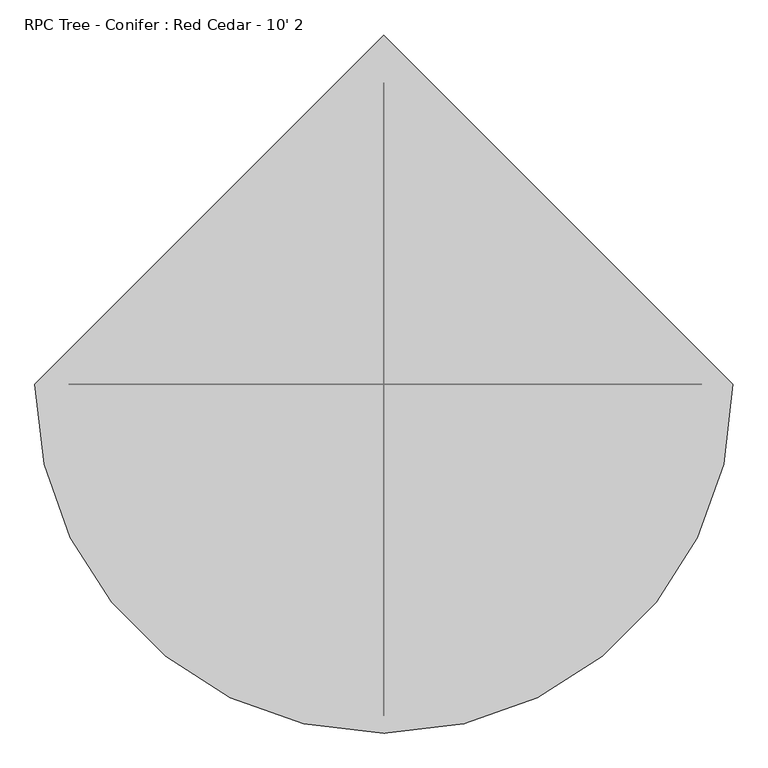
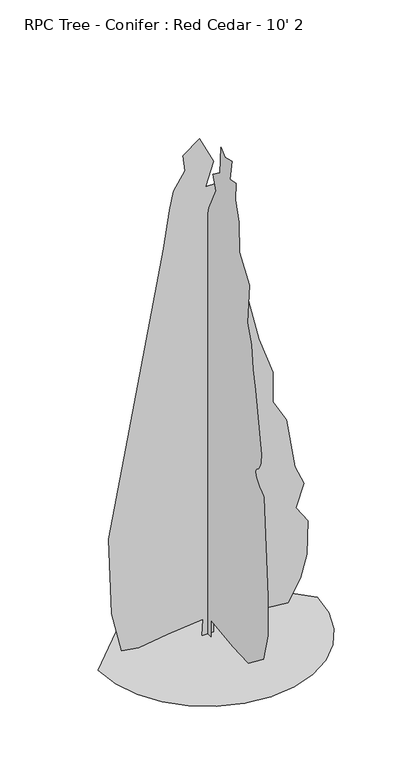
"""IFC4 building model written with IfcOpenShell, lengths in millimetres: geographic element geometry, RPC Tree - Conifer : Red Cedar - 10' 2."""

from ifc_helpers import new_model, si_unit, origin, place, context, project, spatial, triangles, source, transform, mapped, element, save


def rpc_tree_conifer_red_cedar_10_2_15f97043(model_context):
    return source(origin(), model_context, "Body", "Tessellation", [
        triangles([(-83.5718611, 3.7e-06, 7.4e-06), (-70.6343741, -1.16e-05, 245.8064897), (-584.0888028, 1.37e-05, 198.451386), (-999.4580349, 3.55e-05, 137.2780578), (-1247.914381, 4.38e-05, 181.12034), (-1390.2241539, 1.37e-05, 789.1649843), (-1429.0354477, -5.32e-05, 1940.5782063), (-1209.1032326, -0.0001322, 3104.9200722), (-639.8703907, -0.0003352, 6093.4065536), (-549.3098574, -0.0003723, 6649.7173645), (-497.5611992, -0.0003908, 6921.3699692), (-329.3777149, -0.0004136, 7180.132663), (-355.252044, -0.0004263, 7412.9870544), (-122.3830459, -0.0004473, 7594.1527405), (84.6116323, -0.0004317, 7180.132663), (-31.8227487, -0.0004057, 6830.819101), (123.4234529, -0.0004125, 6830.819101), (739.2029903, -0.0002848, 4235.9626625), (938.4659002, -0.0002592, 3661.2180931), (938.4659002, -0.0002322, 3208.4186966), (1132.5218605, -0.0002207, 2872.0531815), (1261.8966671, -0.0001808, 2108.7579117), (1391.2652241, -0.0001688, 1811.2033997), (1274.8316334, -0.0001436, 1474.8377392), (1443.0177338, -0.0001356, 1216.0943756), (1430.0763725, -0.0001049, 711.5426147), (1339.5191093, -8.09e-05, 375.1781533), (1158.3981153, -5.45e-05, 64.6861543), (855.0587093, -4.33e-05, 100.3528226), (433.9154838, -2.44e-05, 90.5604879), (84.6116323, -1.68e-05, 219.9321606), (84.6116323, -3.7e-06, 0.0), (0.1966743, 73.339932, 0.0002301), (0.1966695, 99.2142657, 181.1209758), (0.1966868, 295.5352312, 63.0784626), (0.1966932, 655.5102064, 168.1834843), (0.1966943, 577.8897626, 271.680837), (0.1967153, 1056.5633429, 271.680837), (0.1967266, 1263.5606644, 323.4294951), (0.1967413, 1302.3718128, 620.9846975), (0.196754, 1367.0591434, 1164.3482609), (0.1967591, 1276.4954853, 1371.3391148), (0.1967743, 1289.4368465, 1707.7047752), (0.19678, 1198.8731884, 1927.6369904), (0.1967899, 1160.0619673, 2509.8110481), (0.1967921, 991.8823345, 2729.7432632), (0.1968161, 759.0088308, 3829.4040482), (0.1968294, 500.2661213, 4709.132618), (0.1968359, 319.1464354, 5355.9940063), (0.1968348, 228.5859384, 5420.6755234), (0.1968461, 150.9629329, 5757.0410385), (0.1968576, -30.1575978, 6520.3677017), (0.1968655, -211.2783829, 6882.571756), (0.1968641, -133.6553774, 7089.5817947), (0.1968624, -301.8388799, 7218.9308762), (0.1968788, -327.713209, 7619.9970932), (0.1968703, -431.2105617, 7529.446225), (0.1968647, -599.3933919, 7568.2444382), (0.1968534, -560.5822071, 7270.6835312), (0.1968483, -702.8939421, 7296.5918335), (0.1968375, -689.9526535, 7037.8291397), (0.196835, -780.5163116, 6753.2220932), (0.1968147, -793.4512053, 6300.4038025), (0.1968022, -1047.5908527, 5951.6303238), (0.1967782, -987.5071655, 5343.0529358), (0.1967618, -1091.0057899, 5071.3747513), (0.1967587, -1129.8169384, 4722.0675842), (0.1967434, -1194.5043417, 4437.4544334), (0.1967121, -1336.8141872, 3544.7845024), (0.1967102, -1336.4713303, 3500.4677307), (0.1967083, -1334.0963299, 3456.3733292), (0.1967067, -1327.6448341, 3412.7361671), (0.1967054, -1315.084409, 3369.7786148), (0.1967044, -1294.3770973, 3327.7224609), (0.196704, -1263.4907558, 3286.7967613), (0.1967042, -1220.3805965, 3247.2299904), (0.1967033, -1194.1487675, 3201.3574997), (0.1967003, -1206.8043177, 3145.5030602), (0.196696, -1245.6345783, 3085.8764671), (0.1966912, -1297.9457748, 3028.694783), (0.1966868, -1351.0381737, 2980.155304), (0.1966835, -1392.2051376, 2946.4814873), (0.1966961, -1408.7470058, 2933.8703384), (0.196642, -1504.9938927, 1474.8377392), (0.1966299, -1504.9938927, 879.7286425), (0.1966163, -1388.560302, 452.8011769), (0.1966203, -1013.3834204, 168.1834843), (0.1966378, -625.2671396, 181.12034), (0.1966649, -81.9060743, 258.7433454), (0.1966675, -81.9060743, 0.0002209), (-1583.3149841, 0.0, 0.000295), (-1541.449371, -362.8356654, 0.0002715), (-1422.2281597, -696.0422527, 0.0002465), (-1235.1826, -990.0725613, 0.0002208), (-989.8759163, -1235.379245, 0.0001954), (-695.8456078, -1422.4248047, 0.0001714), (-362.6389841, -1541.6460159, 0.0001497), (0.1967407, -1583.5116291, 0.0001314), (363.0323467, -1541.6460159, 0.000118), (696.2388977, -1422.4248047, 0.0003326), (990.2692062, -1235.379245, 0.0003309), (1235.5822849, -990.0725613, 0.0003348), (1422.6214497, -696.0422527, 0.0001221), (1541.8426609, -362.8356654, 0.0001368), (1583.7082741, 0.0001384, 0.0001566), (0.1964627, 1583.5116291, 0.0003202)], [[13, 14, 15], [12, 13, 15], [12, 15, 16], [11, 12, 16], [32, 1, 2], [31, 32, 2], [10, 11, 16], [16, 17, 18], [10, 16, 18], [9, 10, 18], [8, 9, 18], [8, 18, 19], [8, 19, 20], [7, 8, 20], [7, 20, 21], [7, 21, 22], [6, 7, 22], [6, 22, 23], [6, 23, 24], [5, 6, 24], [4, 5, 24], [3, 4, 24], [2, 3, 24], [31, 2, 24], [30, 31, 24], [29, 30, 24], [29, 24, 25], [29, 25, 26], [29, 26, 27], [29, 27, 28], [55, 56, 57], [35, 36, 37], [57, 58, 59], [55, 57, 59], [59, 60, 61], [89, 90, 33], [89, 33, 34], [53, 54, 55], [55, 59, 61], [53, 55, 61], [53, 61, 62], [52, 53, 62], [52, 62, 63], [51, 52, 63], [51, 63, 64], [51, 64, 65], [50, 51, 65], [38, 39, 40], [34, 35, 37], [50, 65, 66], [50, 66, 67], [49, 50, 67], [48, 49, 67], [48, 67, 68], [47, 48, 68], [47, 68, 69], [46, 47, 69], [46, 69, 70], [46, 70, 71], [46, 71, 72], [46, 72, 73], [46, 73, 74], [46, 74, 75], [46, 75, 76], [46, 76, 77], [46, 77, 78], [46, 78, 79], [46, 79, 80], [37, 38, 40], [37, 40, 41], [37, 41, 42], [46, 80, 81], [82, 83, 84], [34, 37, 42], [89, 34, 42], [89, 42, 43], [89, 43, 44], [45, 46, 81], [44, 45, 81], [89, 44, 81], [88, 89, 81], [88, 81, 82], [88, 82, 84], [88, 84, 85], [88, 85, 86], [88, 86, 87], [105, 106, 91], [104, 105, 91], [104, 91, 92], [103, 104, 92], [103, 92, 93], [103, 93, 94], [102, 103, 94], [101, 102, 94], [101, 94, 95], [101, 95, 96], [101, 96, 97], [101, 97, 98], [101, 98, 99], [101, 99, 100]], closed=False),
    ])


if __name__ == "__main__":
    model = new_model("IFC4")
    model_context = context("Model", 3, world=origin())
    ifc_project = project(units=[si_unit("LENGTHUNIT", "METRE", prefix="MILLI")], contexts=[model_context])
    site = spatial("IfcSite", under=ifc_project)
    building = spatial("IfcBuilding", under=site)
    placement = place(None, origin())
    rpc_tree_conifer_red_cedar_10_2_shape = rpc_tree_conifer_red_cedar_10_2_15f97043(model_context)
    element("IfcGeographicElement", 1, ObjectType="RPC Tree - Conifer : Red Cedar - 10' 2", at=placement, inside=building, context=model_context, shape_type="MappedRepresentation", body=[
        mapped(rpc_tree_conifer_red_cedar_10_2_shape, transform((0.0, 0.0, 0.0), x_axis=(1.0, 0.0, 0.0), y_axis=(0.0, 1.0, 0.0), z_axis=(0.0, 0.0, 1.0))),
    ])
    save(model, "model.ifc")

# Revit data of these elements
# Type "RPC Tree - Conifer : Red Cedar - 10' 2"
#   built-in parameter 1005198 = "{2, 15},{39, RPC-16-FXGH-CPG0-PPQ3-C000-ST1L-LVER-AU},{1, 0},{1, 0},{2, 35},{1, 8},{5, Color},{1, 0},{1, 0},{3, 0.8},{3, 0.8},{3, 0.8},{1, 8},{7, BBoxMin},{1, 0},{1, 0},{1, 0},{1, 0},{1, 0},{1, 8},{7, BBoxMax},{1, 0},{1, 0},{1, 0},{1, 0},{1, 0},{2, 11},{9, RPCTypeId},{1, 0},{1, 0},{39, RPC-16-FXGH-CPG0-PPQ3-C000-ST1L-LVER-AU},{1, 6},{14, RPCPlantHeight},{1, 0},{1, 0},{2, 10},{2, 11},{7, keyword},{1, 0},{1, 0},{99, :Geometry:RPC:Red Cedar:red cedar:western:cupressacae:thuja plicata:north america:evergreen:conifer},{2, 11},{8, category},{1, 0},{1, 0},{16, :Trees [General]},{2, 11},{12, LocalizedUID},{1, 0},{1, 0},{9, Red Cedar},{2, 14},{6, Height},{1, 0},{1, 0},{2, 10},{1, 2},{16, Cast Reflections},{1, 0},{1, 0},{1, 0},{1, 2},{12, Cast Shadows},{1, 0},{1, 0},{1, 1},{1, 2},{9, Lock View},{1, 0},{1, 0},{1, 0},{1, 4},{5, ViewC},{1, 0},{1, 0},{1, 0},{2, 11},{20, AdvancedUIDefinition},{1, 0},{1, 0},{0, },{2, 11},{10, AssetLibID},{1, 0},{1, 0},{36, 4D3F6E72-3F99-4203-98E9-AF80B3C7A7A4},{2, 11},{10, BaseSchema},{1, 0},{1, 0},{9, RPCSchema},{2, 11},{12, ExchangeGUID},{1, 0},{1, 0},{0, },{1, 2},{6, Hidden},{1, 0},{1, 0},{1, 0},{1, 4},{11, RPCCategory},{1, 0},{1, 0},{1, 0},{2, 11},{8, RPCImage},{1, 0},{1, 0},{0, },{1, 4},{13, SchemaVersion},{1, 0},{1, 0},{1, 4},{2, 11},{12, UIDefinition},{1, 0},{1, 0},{0, },{2, 11},{6, UIName},{1, 0},{1, 0},{39, RPC-16-FXGH-CPG0-PPQ3-C000-ST1L-LVER-AU},{2, 11},{11, VersionGUID},{1, 0},{1, 0},{9, RPCSchema},{2, 11},{9, assettype},{1, 0},{1, 0},{11, RPCGeometry},{2, 11},{11, description},{1, 0},{1, 0},{0, },{2, 11},{9, localname},{1, 0},{1, 0},{3, RPC},{2, 11},{9, localtype},{1, 0},{1, 0},{3, RPC},{1, 4},{8, revision},{1, 0},{1, 0},{1, 1},{2, 11},{9, thumbnail},{1, 0},{1, 0},{0, },{1, 4},{7, version},{1, 0},{1, 0},{1, 1},{1, 2},{20, RPC_Cast Reflections},{1, 0},{1, 0},{1, 1},{1, 2},{16, RPC_Cast Shadows},{1, 0},{1, 0},{1, 1},{1, 2},{13, RPC_Lock View},{1, 0},{1, 0},{1, 0},{1, 4},{9, RPC_ViewC},{1, 0},{1, 0},{1, 0},{21, assetlibrary_base.fbx},{1, 5},"
#   built-in parameter 1005195 = "RPC-16-FXGH-CPG0-PPQ3-C000-ST1L-LVER-AU"
#   Type Comments = "Red Cedar"
#   Assembly Code = "G2050500"
#   Height = 25' - 0"
#   Description = (empty or 0)
#   Default Elevation = 0
